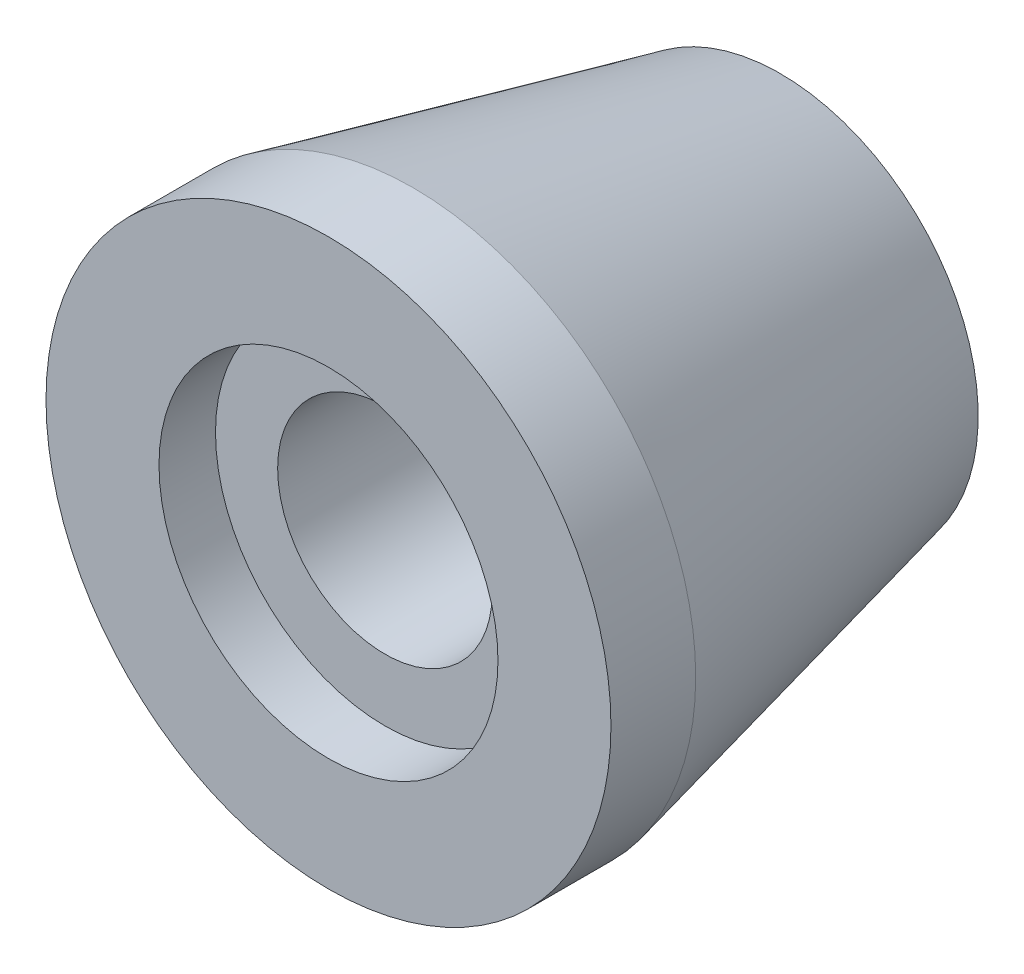
SolidWorks part; units mm, degrees
material "Plain Carbon Steel"
ref_plane "Front Plane" through (0, 0, 0) normal (0, 0, 1) x (1, 0, 0)
ref_plane "Top Plane" through (0, 0, 0) normal (0, 1, 0) x (1, 0, 0)
ref_plane "Right Plane" through (0, 0, 0) normal (1, 0, 0) x (0, 0, -1)
sketch "Bushing Profile Sketch" plane through (0, 0, 0) normal (1, 0, 0) x (0, 0, -1)
  line L0 (0, 17.3385) -> (0, 0) construction
  line L1 (0, 0) -> (-49.8077, 0) construction
  line L9 (0, 3.8) -> (-14, 3.8)
  line L10 (-14, 3.8) -> (-14, 6)
  line L11 (-14, 6) -> (-16, 6)
  line L12 (-16, 6) -> (-16, 10)
  line L13 (-16, 10) -> (-13, 10)
  line L14 (-13, 10) -> (0, 7)
  line L15 (0, 7) -> (0, 3.8)
  dimension "D1" = 7.6
  dimension "D2" = 14
  dimension "D3" = 12
  dimension "D4" = 20
  dimension "D5" = 3
  dimension "D6" = 16
  dimension "D7" = 2
revolve "Bushing Body Revolve" add sketch "Bushing Profile Sketch" angle 360 about L1
